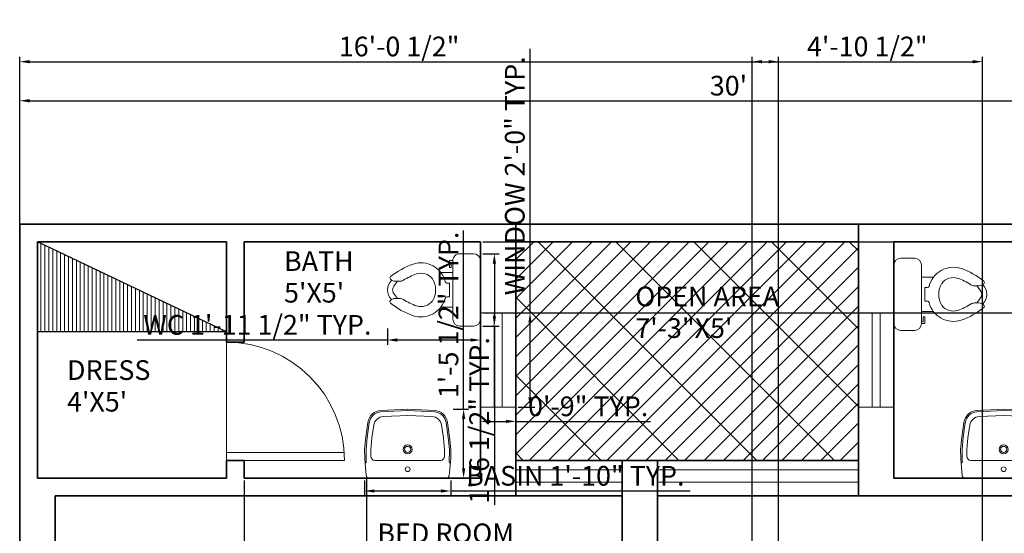
# Model space of a CAD drawing. Units: inches. Extents: x 1265 to 2734, y 1741 to 2595.
# Tile 9 of 10: x 2329 to 2579, y 2464 to 2595. Entities that reach past the tile are written whole.
import ezdxf

# ---------------------------------------------------------------- set-up
doc = ezdxf.new("R2010")
doc.units = ezdxf.units.IN
doc.header["$LTSCALE"] = 0.1
for name, color, linetype, lineweight in [('A-ANNO-DIMS', 2, 'Continuous', 18), ('A-AREA-IDEN', 7, 'Continuous', 18), ('A-DOOR', 3, 'Continuous', 18), ('A-FLOR-CASE', 33, 'Continuous', 25), ('A-FLOR-CASE-PATT', 252, 'Continuous', 13), ('A-FLOR-FIXT', 9, 'Continuous', 18), ('A-FLOR-PATT', 252, 'Continuous', 13), ('A-GLAZ', 4, 'Continuous', 18), ('A-WALL', 7, 'Continuous', 35), ('C-PROP', 7, 'Continuous', 35)]:
    doc.layers.add(name, color=color, linetype=linetype, lineweight=lineweight)
doc.styles.get("Standard").update_dxf_attribs({"font": 'arial.ttf', "height": 5})
doc.dimstyles.new('ISO-25', dxfattribs={"dimtxt": 5, "dimasz": 2.5, "dimexe": 1.25, "dimexo": 0.625, "dimtad": 1, "dimlunit": 3, "dimtxsty": 'Standard', "dimcen": 2.5, "dimadec": 0, "dimazin": 0, "dimtfac": 1, "dimtmove": 0, "dimatfit": 3, "dimfxl": 1, "dimarcsym": 0})

# ---------------------------------------------------------------- blocks, each defined once
blk = doc.blocks.new('*D2')
at = {"layer": 'A-ANNO-DIMS', "color": 0, "lineweight": -2, "transparency": 16777216}
for p, q in [((2328.6, 2543.28), (2328.6, 2575.24)), ((2331.1, 2573.99), (2686.1, 2573.99)), ((2688.6, 2543.28), (2688.6, 2575.24))]:
    blk.add_line(p, q, dxfattribs=at)
at = {"layer": 'A-ANNO-DIMS', "color": 0, "lineweight": 100, "transparency": 16777216}
for points in [[(2331.1, 2574.41), (2331.1, 2573.57), (2328.6, 2573.99)], [(2686.1, 2574.41), (2686.1, 2573.57), (2688.6, 2573.99)]]:
    blk.add_solid(points, dxfattribs=at)
at = {"layer": 'Defpoints', "color": 0, "lineweight": 100, "transparency": 16777216}
for p in [(2688.6, 2573.99), (2328.6, 2542.66), (2688.6, 2542.66)]:
    blk.add_point(p, dxfattribs=at)
at = {"layer": 'A-ANNO-DIMS', "color": 0, "transparency": 16777216, "insert": (2508.6, 2577.17), "char_height": 5, "attachment_point": 5}
blk.add_mtext("30'", dxfattribs=at)
blk = doc.blocks.new('DOOR-SWING-30IN')
for p, q in [((30, 0), (30, 30)), ((0.07, 2), (30, 2)), ((0, 0), (30, 0))]:
    blk.add_line(p, q)
blk.add_arc((30, 0), 30, 90, 180)
blk = doc.blocks.new('WINDOW-24IN')
for p, q in [((9, 24), (0, 24)), ((0, 24), (0, 0)), ((3.5, 24), (3.5, 0)), ((5.5, 24), (5.5, 0)), ((9, 24), (9, 0)), ((9, 0), (0, 0))]:
    blk.add_line(p, q)
blk = doc.blocks.new('WC-FLOOR')
for p, q in [((1.75, 18.37), (5.25, 18.37)), ((0, 1.75), (0, 16.62)), ((7, 16.62), (7, 1.75)), ((10.06, 13.56), (7, 13.56)), ((7.87, 7.44), (7.87, 10.94)), ((7.87, 10.94), (8.54, 10.94)), ((20.5, 11.37), (21.63, 11.37)), ((21.81, 10.35), (21.05, 11.37)), ((21.81, 8.02), (21.05, 7)), ((8.54, 7.44), (7.87, 7.44)), ((20.5, 7), (21.6, 7)), ((10.06, 4.81), (7, 4.81)), ((7.44, 3.5), (7.44, 2.19)), ((7.87, 3.5), (7.44, 3.5)), ((7.87, 1.75), (7.87, 3.5)), ((7.44, 2.19), (7, 2.19)), ((7, 1.75), (7.87, 1.75)), ((5.25, 0), (1.75, 0))]:
    blk.add_line(p, q)
for centre, radius, start, end in [((1.75, 16.62), 1.75, 90, 180), ((5.25, 16.62), 1.75, 0, 90), ((15.09, 9.75), 6.31, 71.8163, 166.1166), ((10.5, -2.84), 19.72, 51.2654, 70.56), ((15.09, 9.75), 3.68, 71.8163, 142.8917), ((10.5, -2.84), 17.09, 57.9375, 70.56), ((22.56, 12.19), 0.437, 314.9399, 51.2654), ((8.54, 11.37), 0.437, 270, 346.1166), ((16.73, 9.19), 5.35, 147.7973, 212.2027), ((20.5, 13.12), 1.75, 237.9375, 270), ((21.63, 13.12), 1.75, 270, 314.9399), ((20.71, 9.19), 1.6, 313.6028, 46.3972), ((20.27, 9.19), 3.35, 313.6028, 46.3972), ((8.54, 7), 0.437, 13.8834, 90), ((15.09, 8.62), 6.31, 193.8834, 288.1837), ((15.09, 8.62), 3.68, 217.1083, 288.1837), ((10.5, 21.22), 17.09, 289.44, 302.0625), ((10.5, 21.22), 19.72, 289.44, 308.665), ((20.5, 5.25), 1.75, 90, 122.0625), ((21.6, 5.25), 1.75, 44.1625, 90), ((22.54, 6.16), 0.437, 308.665, 44.1625), ((1.75, 1.75), 1.75, 180, 270), ((5.25, 1.75), 1.75, 270, 0)]:
    blk.add_arc(centre, radius, start, end)
blk = doc.blocks.new('BASIN-WALL')
for p, q in [((10.93, 17.5), (4.12, 17.17)), ((10.93, 17.15), (4.13, 16.82)), ((10.93, 15.93), (4.76, 15.64)), ((17.75, 17.17), (10.93, 17.5)), ((17.73, 16.82), (10.93, 17.15)), ((17.1, 15.64), (10.93, 15.93)), ((0.84, 14.15), (0.29, 10.37)), ((1.19, 14.1), (0.64, 10.33)), ((2.31, 13.42), (1.84, 10.18)), ((20.02, 10.18), (19.55, 13.42)), ((21.22, 10.33), (20.67, 14.1)), ((21.57, 10.37), (21.02, 14.15)), ((0.29, 10.37), (0, 7.28)), ((0.64, 10.33), (0.35, 7.26)), ((1.84, 10.18), (1.56, 7.21)), ((20.3, 7.21), (20.02, 10.18)), ((21.52, 7.26), (21.22, 10.33)), ((21.86, 7.28), (21.57, 10.37)), ((0, 7.28), (0.02, 4.85)), ((0.35, 7.26), (0.43, 4.17)), ((1.56, 7.21), (1.57, 5.54)), ((20.29, 5.54), (20.3, 7.21)), ((21.43, 4.17), (21.52, 7.26)), ((21.85, 4.85), (21.86, 7.28)), ((0.02, 4.85), (0.4, 0.63)), ((19.25, 4.5), (2.61, 4.5)), ((21.85, 4.85), (21.46, 0.63)), ((20.77, 0), (1.09, 0))]:
    blk.add_line(p, q)
for centre, radius in [((10.93, 7.28), 1.13), ((10.93, 7.28), 0.78), ((10.93, 2.25), 0.606)]:
    blk.add_circle(centre, radius)
for centre, radius, start, end in [((4.28, 13.71), 3.46, 92.7439, 172.7579), ((4.29, 13.7), 3.12, 92.8009, 172.815), ((4.89, 13.04), 2.6, 92.7439, 171.7186), ((16.98, 13.04), 2.6, 8.2775, 87.2561), ((17.58, 13.71), 3.12, 7.2421, 87.2561), ((17.58, 13.71), 3.46, 7.2421, 87.2561), ((2.61, 5.54), 1.04, 180.429, 270), ((19.25, 5.54), 1.04, 270, 359.571), ((0.09, 4.16), 0.346, 275.1819, 0.429), ((21.78, 4.16), 0.346, 179.571, 264.8181), ((1.09, 0.69), 0.693, 185.1819, 270), ((20.77, 0.69), 0.693, 270, 354.8181)]:
    blk.add_arc(centre, radius, start, end)
blk = doc.blocks.new('*D18')
at = {"layer": 'A-ANNO-DIMS', "color": 0, "lineweight": -2, "transparency": 16777216}
for p, q in [((2416.2, 2477.53), (2416.2, 2473.63)), ((2438.06, 2477.53), (2438.06, 2473.63)), ((2418.7, 2474.88), (2435.56, 2474.88)), ((2438.06, 2474.88), (2498.86, 2474.88))]:
    blk.add_line(p, q, dxfattribs=at)
at = {"layer": 'A-ANNO-DIMS', "color": 0, "lineweight": 100, "transparency": 16777216}
for points in [[(2418.7, 2475.29), (2418.7, 2474.46), (2416.2, 2474.88)], [(2435.56, 2475.29), (2435.56, 2474.46), (2438.06, 2474.88)]]:
    blk.add_solid(points, dxfattribs=at)
at = {"layer": 'Defpoints', "color": 0, "lineweight": 100, "transparency": 16777216}
for p in [(2416.2, 2478.16), (2438.06, 2478.16), (2438.06, 2474.88)]:
    blk.add_point(p, dxfattribs=at)
at = {"layer": 'A-ANNO-DIMS', "color": 0, "transparency": 16777216, "insert": (2469.71, 2478.09), "char_height": 5, "attachment_point": 5}
blk.add_mtext('BASIN 1\'-10" TYP.', dxfattribs=at)
blk = doc.blocks.new('*D19')
at = {"layer": 'A-ANNO-DIMS', "color": 0, "lineweight": -2, "transparency": 16777216}
for p, q in [((2441.34, 2495.65), (2441.34, 2541.06)), ((2438.69, 2495.65), (2442.59, 2495.65)), ((2441.34, 2480.66), (2441.34, 2493.15)), ((2438.69, 2478.16), (2442.59, 2478.16))]:
    blk.add_line(p, q, dxfattribs=at)
at = {"layer": 'A-ANNO-DIMS', "color": 0, "lineweight": 100, "transparency": 16777216}
for points in [[(2440.93, 2493.15), (2441.76, 2493.15), (2441.34, 2495.65)], [(2440.93, 2480.66), (2441.76, 2480.66), (2441.34, 2478.16)]]:
    blk.add_solid(points, dxfattribs=at)
at = {"layer": 'Defpoints', "color": 0, "lineweight": 100, "transparency": 16777216}
for p in [(2438.06, 2495.65), (2441.34, 2495.65), (2438.06, 2478.16)]:
    blk.add_point(p, dxfattribs=at)
at = {"layer": 'A-ANNO-DIMS', "color": 0, "transparency": 16777216, "insert": (2438.13, 2519.61), "char_height": 5, "attachment_point": 5, "rotation": 90}
blk.add_mtext('1\'-5 1/2" TYP.', dxfattribs=at)
blk = doc.blocks.new('*D20')
at = {"layer": 'A-ANNO-DIMS', "color": 0, "lineweight": -2, "transparency": 16777216}
for p, q in [((2421.98, 2516.14), (2421.98, 2511.97)), ((2445.6, 2516.14), (2445.6, 2511.97)), ((2421.98, 2513.22), (2358.44, 2513.22)), ((2443.1, 2513.22), (2424.48, 2513.22))]:
    blk.add_line(p, q, dxfattribs=at)
at = {"layer": 'A-ANNO-DIMS', "color": 0, "lineweight": 100, "transparency": 16777216}
for points in [[(2424.48, 2513.64), (2424.48, 2512.8), (2421.98, 2513.22)], [(2443.1, 2513.64), (2443.1, 2512.8), (2445.6, 2513.22)]]:
    blk.add_solid(points, dxfattribs=at)
at = {"layer": 'Defpoints', "color": 0, "lineweight": 100, "transparency": 16777216}
for p in [(2421.98, 2516.76), (2445.6, 2516.76), (2421.98, 2513.22)]:
    blk.add_point(p, dxfattribs=at)
at = {"layer": 'A-ANNO-DIMS', "color": 0, "transparency": 16777216, "insert": (2388.96, 2516.43), "char_height": 5, "attachment_point": 5}
blk.add_mtext('WC 1\'-11 1/2" TYP.', dxfattribs=at)
blk = doc.blocks.new('*D21')
at = {"layer": 'A-ANNO-DIMS', "color": 0, "lineweight": -2, "transparency": 16777216}
for p, q in [((2446.23, 2535.14), (2450.4, 2535.14)), ((2449.15, 2532.64), (2449.15, 2519.26)), ((2446.23, 2516.76), (2450.4, 2516.76)), ((2449.15, 2516.76), (2449.15, 2471.36))]:
    blk.add_line(p, q, dxfattribs=at)
at = {"layer": 'A-ANNO-DIMS', "color": 0, "lineweight": 100, "transparency": 16777216}
for points in [[(2448.73, 2532.64), (2449.56, 2532.64), (2449.15, 2535.14)], [(2448.73, 2519.26), (2449.56, 2519.26), (2449.15, 2516.76)]]:
    blk.add_solid(points, dxfattribs=at)
at = {"layer": 'Defpoints', "color": 0, "lineweight": 100, "transparency": 16777216}
for p in [(2445.6, 2535.14), (2445.6, 2516.76), (2449.15, 2516.76)]:
    blk.add_point(p, dxfattribs=at)
at = {"layer": 'A-ANNO-DIMS', "color": 0, "transparency": 16777216, "insert": (2445.94, 2492.81), "char_height": 5, "attachment_point": 5, "rotation": 90}
blk.add_mtext('1\'-6 1/2" TYP.', dxfattribs=at)
blk = doc.blocks.new('*D22')
at = {"layer": 'A-ANNO-DIMS', "color": 0, "lineweight": -2, "transparency": 16777216}
for p, q in [((2458.2, 2520.16), (2458.2, 2587.18)), ((2455.23, 2520.16), (2459.45, 2520.16)), ((2458.2, 2498.66), (2458.2, 2517.66)), ((2455.23, 2496.16), (2459.45, 2496.16))]:
    blk.add_line(p, q, dxfattribs=at)
at = {"layer": 'A-ANNO-DIMS', "color": 0, "lineweight": 100, "transparency": 16777216}
for points in [[(2457.79, 2517.66), (2458.62, 2517.66), (2458.2, 2520.16)], [(2457.79, 2498.66), (2458.62, 2498.66), (2458.2, 2496.16)]]:
    blk.add_solid(points, dxfattribs=at)
at = {"layer": 'Defpoints', "color": 0, "lineweight": 100, "transparency": 16777216}
for p in [(2454.6, 2520.16), (2458.2, 2520.16), (2454.6, 2496.16)]:
    blk.add_point(p, dxfattribs=at)
at = {"layer": 'A-ANNO-DIMS', "color": 0, "transparency": 16777216, "insert": (2454.99, 2554.92), "char_height": 5, "attachment_point": 5, "rotation": 90}
blk.add_mtext('WINDOW 2\'-0" TYP.', dxfattribs=at)
blk = doc.blocks.new('*D23')
at = {"layer": 'A-ANNO-DIMS', "color": 0, "lineweight": -2, "transparency": 16777216}
for p, q in [((2445.6, 2495.53), (2445.6, 2491.31)), ((2454.6, 2495.53), (2454.6, 2491.31)), ((2448.1, 2492.56), (2452.1, 2492.56)), ((2454.6, 2492.56), (2488.83, 2492.56))]:
    blk.add_line(p, q, dxfattribs=at)
at = {"layer": 'A-ANNO-DIMS', "color": 0, "lineweight": 100, "transparency": 16777216}
for points in [[(2448.1, 2492.97), (2448.1, 2492.14), (2445.6, 2492.56)], [(2452.1, 2492.97), (2452.1, 2492.14), (2454.6, 2492.56)]]:
    blk.add_solid(points, dxfattribs=at)
at = {"layer": 'Defpoints', "color": 0, "lineweight": 100, "transparency": 16777216}
for p in [(2445.6, 2496.16), (2454.6, 2496.16), (2454.6, 2492.56)]:
    blk.add_point(p, dxfattribs=at)
at = {"layer": 'A-ANNO-DIMS', "color": 0, "transparency": 16777216, "insert": (2472.97, 2495.73), "char_height": 5, "attachment_point": 5}
blk.add_mtext('0\'-9" TYP.', dxfattribs=at)
blk = doc.blocks.new('*D42')
at = {"layer": 'A-ANNO-DIMS', "color": 0, "lineweight": -2, "transparency": 16777216}
for p, q in [((2328.6, 1822.68), (2328.6, 2585.16)), ((2331.1, 2583.91), (2518.82, 2583.91)), ((2521.32, 1822.68), (2521.32, 2585.16))]:
    blk.add_line(p, q, dxfattribs=at)
at = {"layer": 'A-ANNO-DIMS', "color": 0, "lineweight": 100, "transparency": 16777216}
for points in [[(2331.1, 2584.32), (2331.1, 2583.49), (2328.6, 2583.91)], [(2518.82, 2584.32), (2518.82, 2583.49), (2521.32, 2583.91)]]:
    blk.add_solid(points, dxfattribs=at)
at = {"layer": 'Defpoints', "color": 0, "lineweight": 100, "transparency": 16777216}
for p in [(2521.32, 2583.91), (2328.6, 1822.06), (2521.32, 1822.06)]:
    blk.add_point(p, dxfattribs=at)
at = {"layer": 'A-ANNO-DIMS', "color": 0, "transparency": 16777216, "insert": (2424.96, 2587.12), "char_height": 5, "attachment_point": 5}
blk.add_mtext('16\'-0 1/2"', dxfattribs=at)
blk = doc.blocks.new('*D44')
at = {"layer": 'A-ANNO-DIMS', "color": 0, "lineweight": -2, "transparency": 16777216}
for p, q in [((2446.23, 2538.16), (2731.1, 2538.16)), ((2729.85, 2535.66), (2729.85, 2522.66)), ((2446.23, 2520.16), (2731.1, 2520.16))]:
    blk.add_line(p, q, dxfattribs=at)
at = {"layer": 'A-ANNO-DIMS', "color": 0, "lineweight": 100, "transparency": 16777216}
for points in [[(2729.44, 2535.66), (2730.27, 2535.66), (2729.85, 2538.16)], [(2729.44, 2522.66), (2730.27, 2522.66), (2729.85, 2520.16)]]:
    blk.add_solid(points, dxfattribs=at)
at = {"layer": 'Defpoints', "color": 0, "lineweight": 100, "transparency": 16777216}
for p in [(2445.6, 2538.16), (2445.6, 2520.16), (2729.85, 2520.16)]:
    blk.add_point(p, dxfattribs=at)
at = {"layer": 'A-ANNO-DIMS', "color": 0, "transparency": 16777216, "insert": (2726.67, 2529.16), "char_height": 5, "attachment_point": 5, "rotation": 90}
blk.add_mtext('1\'-6"', dxfattribs=at)
blk = doc.blocks.new('*D45')
at = {"layer": 'A-ANNO-DIMS', "color": 0, "lineweight": -2, "transparency": 16777216}
for p, q in [((2385.6, 2477.53), (2385.6, 1744.16)), ((2416.67, 2477.91), (2416.67, 1744.16)), ((2388.1, 1745.41), (2414.17, 1745.41))]:
    blk.add_line(p, q, dxfattribs=at)
at = {"layer": 'A-ANNO-DIMS', "color": 0, "lineweight": 100, "transparency": 16777216}
for points in [[(2388.1, 1745.82), (2388.1, 1744.99), (2385.6, 1745.41)], [(2414.17, 1745.82), (2414.17, 1744.99), (2416.67, 1745.41)]]:
    blk.add_solid(points, dxfattribs=at)
at = {"layer": 'Defpoints', "color": 0, "lineweight": 100, "transparency": 16777216}
for p in [(2385.6, 2478.16), (2416.67, 2478.54), (2416.67, 1745.41)]:
    blk.add_point(p, dxfattribs=at)
at = {"layer": 'A-ANNO-DIMS', "color": 0, "transparency": 16777216, "insert": (2401.14, 1748.54), "char_height": 5, "attachment_point": 5}
blk.add_mtext('2\'-7"', dxfattribs=at)
blk = doc.blocks.new('*D47')
at = {"layer": 'A-ANNO-DIMS', "color": 0, "lineweight": -2, "transparency": 16777216}
for p, q in [((2514.6, 1992.78), (2514.6, 2585.16)), ((2517.1, 2583.91), (2570.6, 2583.91)), ((2573.1, 1992.78), (2573.1, 2585.16))]:
    blk.add_line(p, q, dxfattribs=at)
at = {"layer": 'A-ANNO-DIMS', "color": 0, "lineweight": 100, "transparency": 16777216}
for points in [[(2517.1, 2584.32), (2517.1, 2583.49), (2514.6, 2583.91)], [(2570.6, 2584.32), (2570.6, 2583.49), (2573.1, 2583.91)]]:
    blk.add_solid(points, dxfattribs=at)
at = {"layer": 'Defpoints', "color": 0, "lineweight": 100, "transparency": 16777216}
for p in [(2573.1, 2583.91), (2514.6, 1992.16), (2573.1, 1992.16)]:
    blk.add_point(p, dxfattribs=at)
at = {"layer": 'A-ANNO-DIMS', "color": 0, "transparency": 16777216, "insert": (2543.85, 2587.12), "char_height": 5, "attachment_point": 5}
blk.add_mtext('4\'-10 1/2"', dxfattribs=at)

msp = doc.modelspace()

# ---------------------------------------------------------------- hatches: boundary and pattern name
at = {"layer": 'A-FLOR-CASE-PATT'}
h = msp.add_hatch(dxfattribs=at)
h.set_pattern_fill('ANSI31', color=256, scale=0.3149606, angle=45, style=0)
h.paths.add_polyline_path([(2381.102, 2515.307), (2333.102, 2515.307), (2333.102, 2538.157)])
at = {"layer": 'A-FLOR-PATT'}
h = msp.add_hatch(dxfattribs=at)
h.set_pattern_fill('GRATE', color=256, scale=4.4, angle=45)
h.paths.add_polyline_path([(2541.602, 2538.157), (2454.602, 2538.157), (2454.602, 2482.657), (2541.602, 2482.657)])

# ---------------------------------------------------------------- linework, layer by layer
at = {"layer": 'A-FLOR-CASE'}
for q in [(2333.102, 2538.157), (2333.102, 2515.307)]:
    msp.add_line((2381.102, 2515.307), q, dxfattribs=at)
at = {"layer": 'A-GLAZ'}
for p, q in [((2454.602, 2480.231), (2481.602, 2480.231)), ((2490.602, 2480.231), (2541.602, 2480.231)), ((2481.602, 2477.081), (2454.602, 2477.081)), ((2541.602, 2477.081), (2490.602, 2477.081))]:
    msp.add_line(p, q, dxfattribs=at)
at = {"layer": 'A-WALL'}
for p, q in [((2454.602, 2473.657), (2454.602, 2542.657)), ((2541.602, 2473.657), (2541.602, 2542.657)), ((2333.102, 2538.157), (2381.102, 2538.157)), ((2333.102, 2478.157), (2333.102, 2538.157)), ((2381.102, 2512.657), (2381.102, 2538.157)), ((2385.602, 2538.157), (2445.602, 2538.157)), ((2385.602, 2512.657), (2385.602, 2538.157)), ((2445.602, 2478.157), (2445.602, 2538.157)), ((2454.602, 2538.157), (2541.602, 2538.157)), ((2550.602, 2478.157), (2550.602, 2538.157)), ((2550.602, 2538.157), (2622.602, 2538.157)), ((2381.102, 2512.657), (2385.602, 2512.657)), ((2381.102, 2478.157), (2381.102, 2482.657)), ((2381.102, 2482.657), (2385.602, 2482.657)), ((2385.602, 2478.157), (2385.602, 2482.657)), ((2454.602, 2482.657), (2541.602, 2482.657)), ((2481.602, 2317.657), (2481.602, 2482.657)), ((2490.602, 2317.657), (2490.602, 2482.657)), ((2333.102, 2478.157), (2381.102, 2478.157)), ((2385.602, 2478.157), (2445.602, 2478.157)), ((2550.602, 2478.157), (2622.602, 2478.157)), ((2337.602, 2473.657), (2481.602, 2473.657)), ((2337.602, 2317.657), (2337.602, 2473.657)), ((2490.602, 2473.657), (2631.602, 2473.657))]:
    msp.add_line(p, q, dxfattribs=at)
at = {"layer": 'C-PROP'}
for p, q in [((2328.602, 2542.657), (2688.602, 2542.657)), ((2328.602, 1786.657), (2328.602, 2542.657))]:
    msp.add_line(p, q, dxfattribs=at)

# ---------------------------------------------------------------- block references
at = {"layer": 'A-DOOR', "extrusion": (0, 0, -1), "zscale": -1}
msp.add_blockref('DOOR-SWING-30IN', (-2411.103, 2482.657), dxfattribs=at)
at = {"layer": 'A-FLOR-FIXT', "rotation": 180}
msp.add_blockref('WC-FLOOR', (2445.603, 2535.137), dxfattribs=at)
at = {"layer": 'A-FLOR-FIXT'}
for name, p in [('WC-FLOOR', (2550.602, 2515.633)), ('BASIN-WALL', (2416.201, 2478.157)), ('BASIN-WALL', (2567.559, 2478.157))]:
    msp.add_blockref(name, p, dxfattribs=at)
at = {"layer": 'A-GLAZ'}
msp.add_blockref('WINDOW-24IN', (2445.602, 2496.157), dxfattribs=at)
at = {"layer": 'A-GLAZ', "rotation": 180}
msp.add_blockref('WINDOW-24IN', (2550.603, 2520.156), dxfattribs=at)

# ---------------------------------------------------------------- texts
at = {"layer": 'A-AREA-IDEN'}
for s, p in [('BATH', (2395.736, 2530.763)), ("5'X5'", (2395.736, 2522.731)), ('OPEN AREA', (2484.942, 2521.782)), ('7\'-3"X5\'', (2484.942, 2513.75)), ('DRESS', (2340.625, 2503.087)), ("4'X5'", (2340.625, 2495.055)), ('BED ROOM', (2419.434, 2461.629))]:
    msp.add_text(s, height=5, dxfattribs=at).set_placement(p)

# ---------------------------------------------------------------- dimensions: what is measured, and where the dimension line sits
at = {"layer": 'A-ANNO-DIMS'}
for base, p1, p2, override, picture, middle in [((2521.319, 2583.907), (2328.602, 1822.059), (2521.319, 1822.059), {"dimdec": 1, "dimlfac": 1, "dimrnd": 0, "dimzin": 1, "dimdsep": 46, "dimlunit": 4, "dimfrac": 2}, '*D42', (2424.961, 2587.117)), ((2573.102, 2583.907), (2514.602, 1992.157), (2573.102, 1992.157), {"dimdec": 1, "dimlfac": 1, "dimrnd": 0, "dimzin": 1, "dimdsep": 46, "dimlunit": 4, "dimfrac": 2}, '*D47', (2543.852, 2587.117)), ((2688.602, 2573.99), (2328.602, 2542.657), (2688.602, 2542.657), {"dimclrd": 0, "dimclre": 0, "dimclrt": 0}, '*D2', (2508.602, 2577.169)), ((2416.673, 1745.407), (2385.602, 2478.157), (2416.673, 2478.538), {"dimdec": 1, "dimlfac": 1, "dimrnd": 0, "dimzin": 1, "dimdsep": 46, "dimlunit": 4, "dimfrac": 2}, '*D45', (2401.138, 1748.542))]:
    dim = msp.add_linear_dim(base=base, p1=p1, p2=p2, dimstyle='ISO-25', override=override, dxfattribs=at)
    dim.commit()
    dim.dimension.update_dxf_attribs({"geometry": picture, "text_midpoint": middle})
for base, p1, p2, angle, text, picture, middle in [((2458.202, 2520.157), (2454.602, 2496.157), (2454.602, 2520.157), 90, 'WINDOW <> TYP.', '*D22', (2454.99, 2554.917)), ((2441.343, 2495.653), (2438.064, 2478.157), (2438.064, 2495.653), 90, '<> TYP.', '*D19', (2438.133, 2519.607)), ((2449.146, 2516.765), (2445.602, 2535.138), (2445.602, 2516.765), 270, '<> TYP.', '*D21', (2445.935, 2492.811)), ((2421.98, 2513.222), (2445.602, 2516.765), (2421.98, 2516.765), 180, 'WC <> TYP.', '*D20', (2388.958, 2516.432))]:
    dim = msp.add_linear_dim(base=base, p1=p1, p2=p2, angle=angle, text=text, dimstyle='ISO-25', override={"dimdec": 1, "dimlfac": 1, "dimrnd": 0, "dimzin": 1, "dimdsep": 46, "dimlunit": 4, "dimfrac": 2}, dxfattribs=at)
    dim.commit()
    dim.dimension.update_dxf_attribs({"geometry": picture, "text_midpoint": middle})
dim = msp.add_linear_dim(base=(2729.852, 2520.157), p1=(2445.602, 2538.157), p2=(2445.602, 2520.157), angle=90, dimstyle='ISO-25', override={"dimdec": 1, "dimlfac": 1, "dimrnd": 0, "dimzin": 1, "dimdsep": 46, "dimlunit": 4, "dimfrac": 2}, dxfattribs=at)
dim.commit()
dim.dimension.update_dxf_attribs({"geometry": '*D44', "text_midpoint": (2726.675, 2529.157)})
for base, p1, p2, text, picture, middle in [((2454.602, 2492.557), (2445.602, 2496.157), (2454.602, 2496.157), '<> TYP.', '*D23', (2472.966, 2495.735)), ((2438.064, 2474.877), (2416.201, 2478.157), (2438.064, 2478.157), 'BASIN <> TYP.', '*D18', (2469.71, 2478.088))]:
    dim = msp.add_linear_dim(base=base, p1=p1, p2=p2, text=text, dimstyle='ISO-25', override={"dimdec": 1, "dimlfac": 1, "dimrnd": 0, "dimzin": 1, "dimdsep": 46, "dimlunit": 4, "dimfrac": 2}, dxfattribs=at)
    dim.commit()
    dim.dimension.update_dxf_attribs({"geometry": picture, "text_midpoint": middle})

doc.saveas('drawing.dxf')
